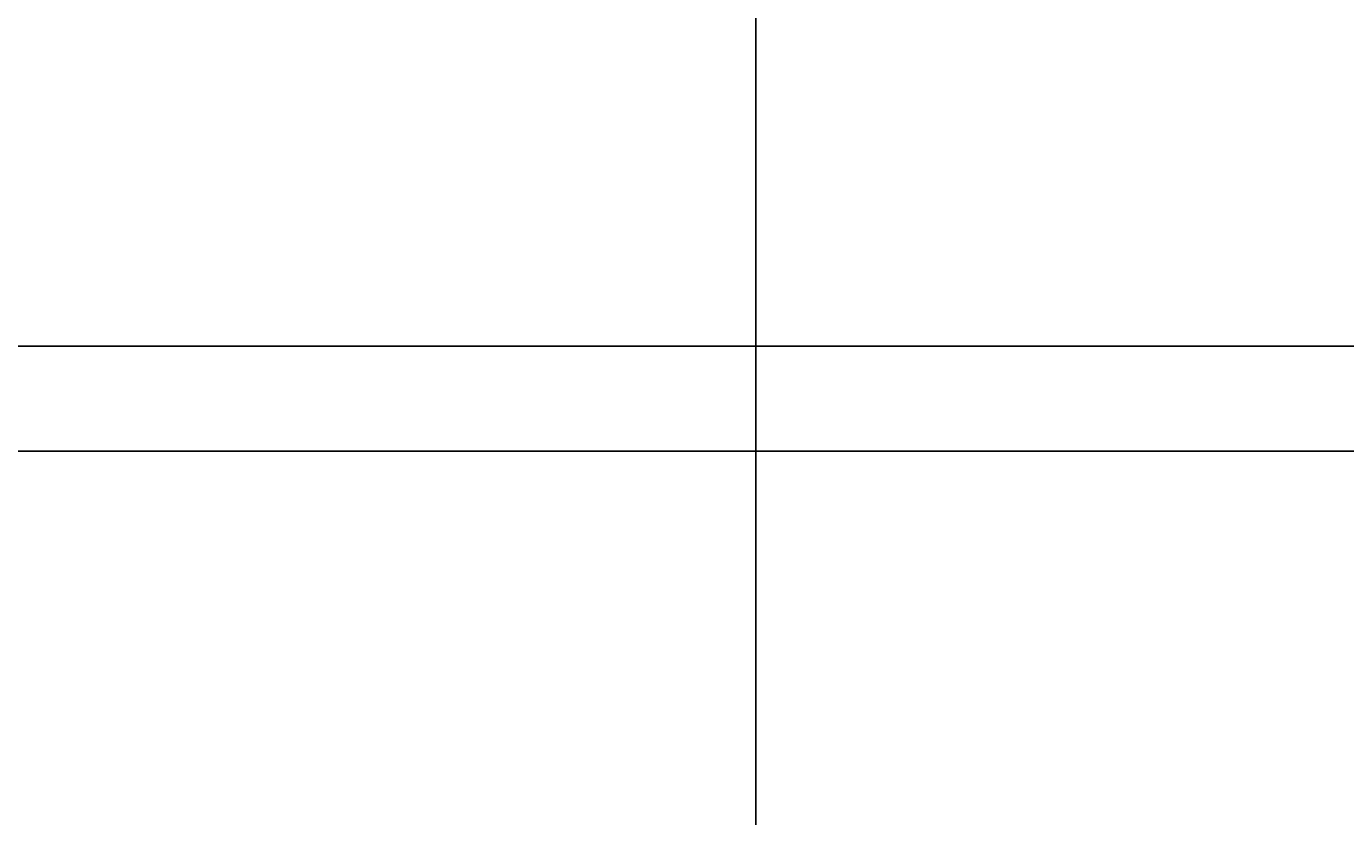
# Model space of a CAD drawing. Units: inches. Extents: x 35362 to 73946, y 43607 to 67532.
# Tile 86 of 134: x 51337 to 52380, y 46919 to 47544. Entities that reach past the tile are written whole.
import ezdxf

# ---------------------------------------------------------------- set-up
doc = ezdxf.new("R2010")
doc.units = ezdxf.units.IN
doc.header["$MEASUREMENT"] = 0
doc.layers.add('A-ANNO-DIMS', color=2, linetype='Continuous', lineweight=18)
doc.styles.get("Standard").update_dxf_attribs({"font": 'arial.ttf'})
doc.dimstyles.get("Standard").update_dxf_attribs({"dimtxt": 0.18, "dimasz": 0.18, "dimexe": 0.18, "dimexo": 0.0625, "dimgap": 0.09, "dimtad": 0, "dimtih": 1, "dimtoh": 1, "dimdec": 4, "dimzin": 0, "dimdsep": 46, "dimtxsty": 'Standard', "dimcen": 0.09, "dimadec": 0, "dimazin": 0, "dimtfac": 1, "dimtdec": 4, "dimtofl": 0, "dimtmove": 0, "dimatfit": 3, "dimfxl": 1, "dimtolj": 1, "dimtzin": 0, "dimarcsym": 0})

# ---------------------------------------------------------------- blocks, each defined once
blk = doc.blocks.new('*D11')
at = {"layer": 'A-ANNO-DIMS', "color": 0, "lineweight": -2, "transparency": 16777216}
for p, q in [((47978.7, 56028.8), (47978.7, 43606.7)), ((53109.8, 56028.8), (53109.8, 43606.7)), ((47978.8, 43606.9), (50543.9, 43606.9)), ((53109.6, 43606.9), (50544.6, 43606.9))]:
    blk.add_line(p, q, dxfattribs=at)
at = {"layer": 'A-ANNO-DIMS', "color": 0, "transparency": 16777216}
for points in [[(47978.8, 43606.9), (47978.8, 43606.8), (47978.7, 43606.9)], [(53109.6, 43606.9), (53109.6, 43606.8), (53109.8, 43606.9)]]:
    blk.add_solid(points, dxfattribs=at)
at = {"layer": 'Defpoints', "color": 0, "transparency": 16777216}
for p in [(47978.7, 56028.8), (53109.8, 56028.8), (53109.8, 43606.9)]:
    blk.add_point(p, dxfattribs=at)
at = {"layer": 'A-ANNO-DIMS', "color": 0, "transparency": 16777216, "insert": (50544.2, 43606.9), "char_height": 0.18, "attachment_point": 5}
blk.add_mtext('\\A1;5131', dxfattribs=at)
blk = doc.blocks.new('*D17')
at = {"layer": 'A-ANNO-DIMS', "color": 0, "lineweight": -2, "transparency": 16777216}
for p, q in [((49923.3, 61293.2), (49923.3, 43606.7)), ((51913.9, 61293.2), (51913.9, 43606.7)), ((49923.5, 43606.9), (50918.2, 43606.9)), ((51913.8, 43606.9), (50919.1, 43606.9))]:
    blk.add_line(p, q, dxfattribs=at)
at = {"layer": 'A-ANNO-DIMS', "color": 0, "transparency": 16777216}
for points in [[(49923.5, 43606.9), (49923.5, 43606.8), (49923.3, 43606.9)], [(51913.8, 43606.9), (51913.8, 43606.8), (51913.9, 43606.9)]]:
    blk.add_solid(points, dxfattribs=at)
at = {"layer": 'Defpoints', "color": 0, "transparency": 16777216}
for p in [(49923.3, 61293.3), (51913.9, 61293.3), (51913.9, 43606.9)]:
    blk.add_point(p, dxfattribs=at)
at = {"layer": 'A-ANNO-DIMS', "color": 0, "transparency": 16777216, "insert": (50918.6, 43606.9), "char_height": 0.18, "attachment_point": 5}
blk.add_mtext('\\A1;1990.6', dxfattribs=at)
blk = doc.blocks.new('*D43')
at = {"layer": 'A-ANNO-DIMS', "color": 0, "lineweight": -2, "transparency": 16777216}
for p, q in [((62004.7, 47625.2), (35361.8, 47625.2)), ((35361.9, 47625), (35361.9, 47416.9)), ((35361.9, 47208.4), (35361.9, 47416.5)), ((62004.7, 47208.2), (35361.8, 47208.2))]:
    blk.add_line(p, q, dxfattribs=at)
at = {"layer": 'A-ANNO-DIMS', "color": 0, "transparency": 16777216}
for points in [[(35361.9, 47625), (35362, 47625), (35361.9, 47625.2)], [(35361.9, 47208.4), (35362, 47208.4), (35361.9, 47208.2)]]:
    blk.add_solid(points, dxfattribs=at)
at = {"layer": 'Defpoints', "color": 0, "transparency": 16777216}
for p in [(62004.7, 47625.2), (35361.9, 47208.2), (62004.7, 47208.2)]:
    blk.add_point(p, dxfattribs=at)
at = {"layer": 'A-ANNO-DIMS', "color": 0, "transparency": 16777216, "insert": (35361.9, 47416.7), "char_height": 0.18, "attachment_point": 5}
blk.add_mtext('\\A1;416.9', dxfattribs=at)
blk = doc.blocks.new('*D67')
at = {"layer": 'A-ANNO-DIMS', "color": 0, "lineweight": -2, "transparency": 16777216}
for p, q in [((56873.5, 53351.5), (35361.8, 53351.5)), ((35361.9, 53351.3), (35361.9, 49400.9)), ((35361.9, 45450.1), (35361.9, 49400.5)), ((53793.6, 45449.9), (35361.8, 45449.9))]:
    blk.add_line(p, q, dxfattribs=at)
at = {"layer": 'A-ANNO-DIMS', "color": 0, "transparency": 16777216}
for points in [[(35361.9, 53351.3), (35362, 53351.3), (35361.9, 53351.5)], [(35361.9, 45450.1), (35362, 45450.1), (35361.9, 45449.9)]]:
    blk.add_solid(points, dxfattribs=at)
at = {"layer": 'Defpoints', "color": 0, "transparency": 16777216}
for p in [(35361.9, 53351.5), (56873.6, 53351.5), (53793.6, 45449.9)]:
    blk.add_point(p, dxfattribs=at)
at = {"layer": 'A-ANNO-DIMS', "color": 0, "transparency": 16777216, "insert": (35361.9, 49400.7), "char_height": 0.18, "attachment_point": 5}
blk.add_mtext('\\A1;7901.6', dxfattribs=at)
blk = doc.blocks.new('*D90')
at = {"layer": 'A-ANNO-DIMS', "color": 0, "lineweight": -2, "transparency": 16777216}
for p, q in [((53707.7, 47291.3), (35361.8, 47291.3)), ((35361.9, 47291.1), (35361.9, 46710.3)), ((35361.9, 46129.1), (35361.9, 46709.9)), ((53793.6, 46128.9), (35361.8, 46128.9))]:
    blk.add_line(p, q, dxfattribs=at)
at = {"layer": 'A-ANNO-DIMS', "color": 0, "transparency": 16777216}
for points in [[(35361.9, 47291.1), (35362, 47291.1), (35361.9, 47291.3)], [(35361.9, 46129.1), (35362, 46129.1), (35361.9, 46128.9)]]:
    blk.add_solid(points, dxfattribs=at)
at = {"layer": 'Defpoints', "color": 0, "transparency": 16777216}
for p in [(53707.8, 47291.3), (35361.9, 46128.9), (53793.6, 46128.9)]:
    blk.add_point(p, dxfattribs=at)
at = {"layer": 'A-ANNO-DIMS', "color": 0, "transparency": 16777216, "insert": (35361.9, 46710.1), "char_height": 0.18, "attachment_point": 5}
blk.add_mtext('\\A1;1162.4', dxfattribs=at)

msp = doc.modelspace()

# ---------------------------------------------------------------- dimensions: what is measured, and where the dimension line sits
at = {"layer": 'A-ANNO-DIMS'}
for base, p1, p2, override, picture, middle in [((51913.931, 43606.859), (49923.307, 61293.286), (51913.931, 61293.286), {"dimdec": 1, "dimlfac": 1, "dimrnd": 0, "dimzin": 0, "dimdsep": 46, "dimlunit": 2}, '*D17', (50918.619, 43606.859)), ((53109.76, 43606.859), (47978.665, 56028.836), (53109.76, 56028.836), {"dimdec": 0, "dimlfac": 1, "dimrnd": 0, "dimzin": 0, "dimdsep": 46, "dimlunit": 2}, '*D11', (50544.212, 43606.859))]:
    dim = msp.add_linear_dim(base=base, p1=p1, p2=p2, dimstyle='Standard', override=override, dxfattribs=at)
    dim.commit()
    dim.dimension.update_dxf_attribs({"geometry": picture, "text_midpoint": middle})
for base, p1, p2, picture, middle in [((35361.949, 53351.529), (53793.638, 45449.894), (56873.602, 53351.529), '*D67', (35361.949, 49400.712)), ((35361.949, 47208.25), (62004.728, 47625.181), (62004.728, 47208.25), '*D43', (35361.949, 47416.715)), ((35361.949, 46128.878), (53707.781, 47291.285), (53793.638, 46128.878), '*D90', (35361.949, 46710.081))]:
    dim = msp.add_linear_dim(base=base, p1=p1, p2=p2, angle=90, dimstyle='Standard', override={"dimdec": 1, "dimlfac": 1, "dimrnd": 0, "dimzin": 0, "dimdsep": 46, "dimlunit": 2}, dxfattribs=at)
    dim.commit()
    dim.dimension.update_dxf_attribs({"geometry": picture, "text_midpoint": middle})

doc.saveas('drawing.dxf')
